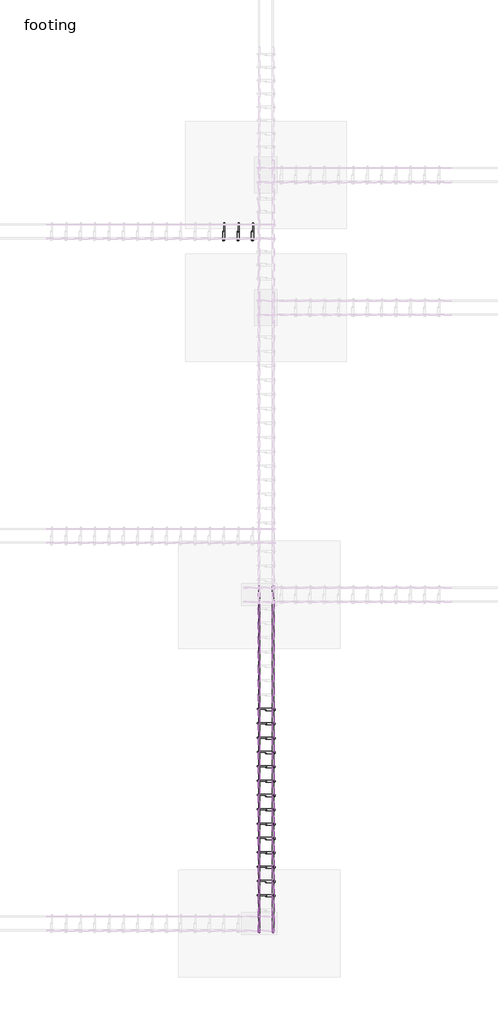
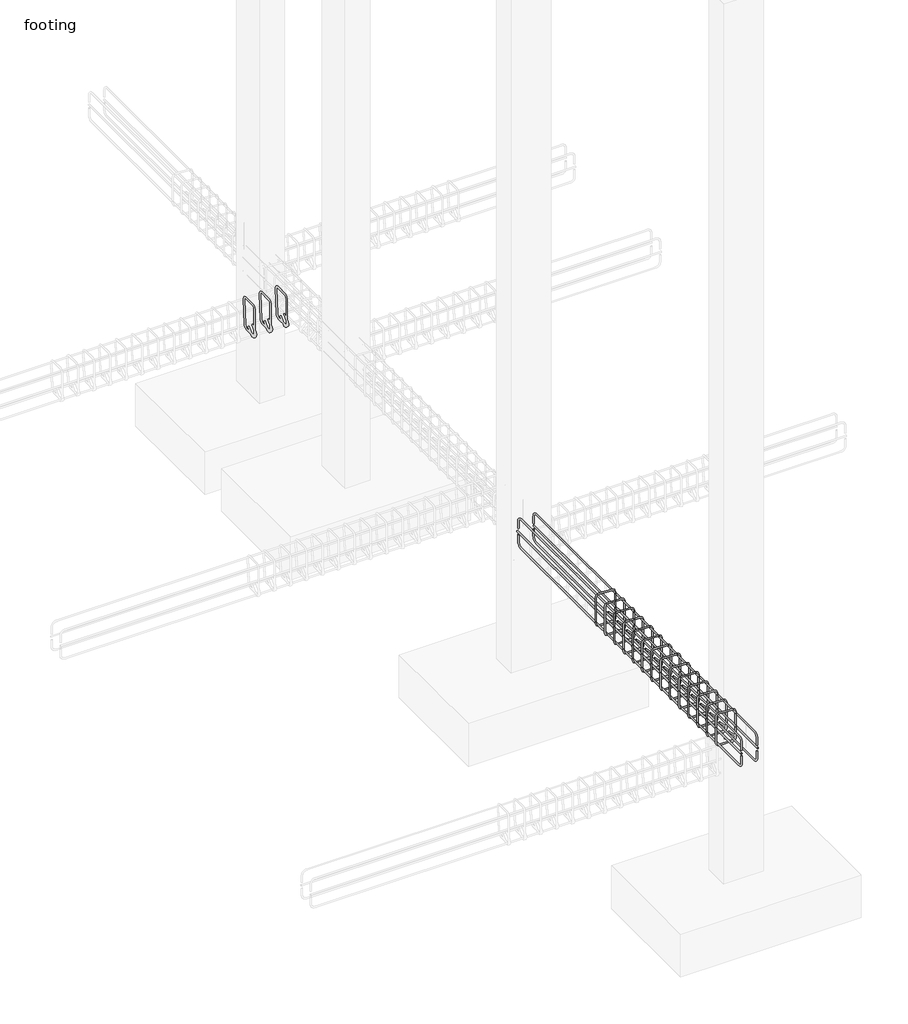
# One storey, part 9 of 21: 23 reinforcing bars.
"""IFC4 building model written with IfcOpenShell, lengths in millimetres."""

from ifc_helpers import new_model, si_unit, point, frame, origin, place, context, project, spatial, polyline, circle_curve, trimmed, segment, composite_curve, element, save
from ifc_brep_helpers import swept_disk

model = new_model("IFC4")

# Units and contexts
model_context = context("Model", 3, world=origin())
ifc_project = project(units=[si_unit("LENGTHUNIT", "METRE", prefix="MILLI")], contexts=[model_context])

# Site, building, storey
site = spatial("IfcSite", under=ifc_project)
building = spatial("IfcBuilding", under=site)
storey = spatial("IfcBuildingStorey", under=building, Name="footing", Elevation=-1524.0)

# Reinforcing bars
placement = place(None, origin())
element("IfcReinforcingBar", 1, at=placement, inside=storey, context=model_context, shape_type="SolidModel", body=[
    swept_disk(composite_curve([segment(polyline([(-8352.8883428, 7572.2887132, -310.8825168), (-8352.8883428, 7517.4237147, -365.7475153)]), True, "CONTINUOUS"), segment(trimmed(circle_curve(frame((-8352.8883428, 7494.9730744, -343.296875), z_axis=(-1.0, 0.0, 0.0), x_axis=(0.0, 22.450640300000487, -22.450640299999975)), 31.75), [point((-8352.8883428, 7517.4237147, -365.7475153))], [point((-8352.8883428, 7463.2230744, -343.296875))], True, "CARTESIAN"), True, "CONTINUOUS"), segment(polyline([(-8352.8883428, 7463.2230744, -343.296875), (-8352.8883428, 7463.2230744, -63.103125)]), True, "CONTINUOUS"), segment(trimmed(circle_curve(frame((-8352.8883428, 7494.9730744, -63.103125), z_axis=(-1.0, 0.0, 0.0), x_axis=(0.0, -31.75, 0.0)), 31.75), [point((-8352.8883428, 7463.2230744, -63.103125))], [point((-8352.8883428, 7494.9730744, -31.353125))], True, "CARTESIAN"), True, "CONTINUOUS"), segment(polyline([(-8352.8883428, 7494.9730744, -31.353125), (-8352.8883428, 7622.7668244, -31.353125)]), True, "CONTINUOUS"), segment(trimmed(circle_curve(frame((-8351.7159328, 7622.7668244, -63.0814712), z_axis=(-0.9993179916193466, 0.0, -0.03692629992126919), x_axis=(-1.1724100000010367, 0.0, 31.728346200000004)), 31.75), [point((-8352.8883428, 7622.7668244, -31.353125))], [point((-8351.7159328, 7654.5168244, -63.0814712))], True, "CARTESIAN"), True, "CONTINUOUS"), segment(polyline([(-8351.7159328, 7654.5168244, -63.0814712), (-8341.3607528, 7654.5168244, -343.3185288)]), True, "CONTINUOUS"), segment(trimmed(circle_curve(frame((-8341.3607528, 7622.7668244, -343.3185288), z_axis=(-0.9993179916193466, 0.0, -0.03692629992126919), x_axis=(0.0, 31.75, 0.0)), 31.75), [point((-8341.3607528, 7654.5168244, -343.3185288))], [point((-8340.1883428, 7622.7668244, -375.046875))], True, "CARTESIAN"), True, "CONTINUOUS"), segment(polyline([(-8340.1883428, 7622.7668244, -375.046875), (-8340.1883428, 7494.9730744, -375.046875)]), True, "CONTINUOUS"), segment(trimmed(circle_curve(frame((-8340.1883428, 7494.9730744, -343.296875), z_axis=(-1.0, 0.0, 0.0), x_axis=(0.0, 0.0, -31.75)), 31.75), [point((-8340.1883428, 7494.9730744, -375.046875))], [point((-8340.1883428, 7472.5224341, -320.8462347))], True, "CARTESIAN"), True, "CONTINUOUS"), segment(polyline([(-8340.1883428, 7472.5224341, -320.8462347), (-8340.1883428, 7527.3874326, -265.9812362)]), True, "CONTINUOUS")], self_intersect=False), 6.35),
])
element("IfcReinforcingBar", 2, at=placement, inside=storey, context=model_context, shape_type="SolidModel", body=[
    swept_disk(composite_curve([segment(polyline([(-8190.1883428, 7572.2887132, -310.8825168), (-8190.1883428, 7517.4237147, -365.7475153)]), True, "CONTINUOUS"), segment(trimmed(circle_curve(frame((-8190.1883428, 7494.9730744, -343.296875), z_axis=(-1.0, 0.0, 0.0), x_axis=(0.0, 22.450640300000487, -22.450640299999975)), 31.75), [point((-8190.1883428, 7517.4237147, -365.7475153))], [point((-8190.1883428, 7463.2230744, -343.296875))], True, "CARTESIAN"), True, "CONTINUOUS"), segment(polyline([(-8190.1883428, 7463.2230744, -343.296875), (-8190.1883428, 7463.2230744, -63.103125)]), True, "CONTINUOUS"), segment(trimmed(circle_curve(frame((-8190.1883428, 7494.9730744, -63.103125), z_axis=(-1.0, 0.0, 0.0), x_axis=(0.0, -31.75, 0.0)), 31.75), [point((-8190.1883428, 7463.2230744, -63.103125))], [point((-8190.1883428, 7494.9730744, -31.353125))], True, "CARTESIAN"), True, "CONTINUOUS"), segment(polyline([(-8190.1883428, 7494.9730744, -31.353125), (-8190.1883428, 7622.7668244, -31.353125)]), True, "CONTINUOUS"), segment(trimmed(circle_curve(frame((-8189.0159328, 7622.7668244, -63.0814712), z_axis=(-0.9993179916193466, 0.0, -0.03692629992126919), x_axis=(-1.1724100000001272, 0.0, 31.728346200000004)), 31.75), [point((-8190.1883428, 7622.7668244, -31.353125))], [point((-8189.0159328, 7654.5168244, -63.0814712))], True, "CARTESIAN"), True, "CONTINUOUS"), segment(polyline([(-8189.0159328, 7654.5168244, -63.0814712), (-8178.6607528, 7654.5168244, -343.3185288)]), True, "CONTINUOUS"), segment(trimmed(circle_curve(frame((-8178.6607528, 7622.7668244, -343.3185288), z_axis=(-0.9993179916193466, 0.0, -0.03692629992126919), x_axis=(0.0, 31.75, 0.0)), 31.75), [point((-8178.6607528, 7654.5168244, -343.3185288))], [point((-8177.4883428, 7622.7668244, -375.046875))], True, "CARTESIAN"), True, "CONTINUOUS"), segment(polyline([(-8177.4883428, 7622.7668244, -375.046875), (-8177.4883428, 7494.9730744, -375.046875)]), True, "CONTINUOUS"), segment(trimmed(circle_curve(frame((-8177.4883428, 7494.9730744, -343.296875), z_axis=(-1.0, 0.0, 0.0), x_axis=(0.0, 0.0, -31.75)), 31.75), [point((-8177.4883428, 7494.9730744, -375.046875))], [point((-8177.4883428, 7472.5224341, -320.8462347))], True, "CARTESIAN"), True, "CONTINUOUS"), segment(polyline([(-8177.4883428, 7472.5224341, -320.8462347), (-8177.4883428, 7527.3874326, -265.9812362)]), True, "CONTINUOUS")], self_intersect=False), 6.35),
])
element("IfcReinforcingBar", 3, at=placement, inside=storey, context=model_context, shape_type="SolidModel", body=[
    swept_disk(composite_curve([segment(polyline([(-8027.4883428, 7572.2887132, -310.8825168), (-8027.4883428, 7517.4237147, -365.7475153)]), True, "CONTINUOUS"), segment(trimmed(circle_curve(frame((-8027.4883428, 7494.9730744, -343.296875), z_axis=(-1.0, 0.0, 0.0), x_axis=(0.0, 22.450640300000487, -22.450640299999975)), 31.75), [point((-8027.4883428, 7517.4237147, -365.7475153))], [point((-8027.4883428, 7463.2230744, -343.296875))], True, "CARTESIAN"), True, "CONTINUOUS"), segment(polyline([(-8027.4883428, 7463.2230744, -343.296875), (-8027.4883428, 7463.2230744, -63.103125)]), True, "CONTINUOUS"), segment(trimmed(circle_curve(frame((-8027.4883428, 7494.9730744, -63.103125), z_axis=(-1.0, 0.0, 0.0), x_axis=(0.0, -31.75, 0.0)), 31.75), [point((-8027.4883428, 7463.2230744, -63.103125))], [point((-8027.4883428, 7494.9730744, -31.353125))], True, "CARTESIAN"), True, "CONTINUOUS"), segment(polyline([(-8027.4883428, 7494.9730744, -31.353125), (-8027.4883428, 7622.7668244, -31.353125)]), True, "CONTINUOUS"), segment(trimmed(circle_curve(frame((-8026.3159328, 7622.7668244, -63.0814712), z_axis=(-0.9993179916193466, 0.0, -0.03692629992126919), x_axis=(-1.1724100000001272, 0.0, 31.728346200000004)), 31.75), [point((-8027.4883428, 7622.7668244, -31.353125))], [point((-8026.3159328, 7654.5168244, -63.0814712))], True, "CARTESIAN"), True, "CONTINUOUS"), segment(polyline([(-8026.3159328, 7654.5168244, -63.0814712), (-8015.9607528, 7654.5168244, -343.3185288)]), True, "CONTINUOUS"), segment(trimmed(circle_curve(frame((-8015.9607528, 7622.7668244, -343.3185288), z_axis=(-0.9993179916193466, 0.0, -0.03692629992126919), x_axis=(0.0, 31.75, 0.0)), 31.75), [point((-8015.9607528, 7654.5168244, -343.3185288))], [point((-8014.7883428, 7622.7668244, -375.046875))], True, "CARTESIAN"), True, "CONTINUOUS"), segment(polyline([(-8014.7883428, 7622.7668244, -375.046875), (-8014.7883428, 7494.9730744, -375.046875)]), True, "CONTINUOUS"), segment(trimmed(circle_curve(frame((-8014.7883428, 7494.9730744, -343.296875), z_axis=(-1.0, 0.0, 0.0), x_axis=(0.0, 0.0, -31.75)), 31.75), [point((-8014.7883428, 7494.9730744, -375.046875))], [point((-8014.7883428, 7472.5224341, -320.8462347))], True, "CARTESIAN"), True, "CONTINUOUS"), segment(polyline([(-8014.7883428, 7472.5224341, -320.8462347), (-8014.7883428, 7527.3874326, -265.9812362)]), True, "CONTINUOUS")], self_intersect=False), 6.35),
])
element("IfcReinforcingBar", 4, at=placement, inside=storey, context=model_context, shape_type="SolidModel", body=[
    swept_disk(composite_curve([segment(polyline([(-7834.7165254, 26.8956073, -265.9812362), (-7779.851527, 26.8956073, -320.8462347)]), True, "CONTINUOUS"), segment(trimmed(circle_curve(frame((-7802.3021673, 26.8956073, -343.296875), z_axis=(0.0, 1.0, 0.0), x_axis=(22.450640300000487, 0.0, 22.450640299999975)), 31.75), [point((-7779.851527, 26.8956073, -320.8462347))], [point((-7802.3021673, 26.8956073, -375.046875))], True, "CARTESIAN"), True, "CONTINUOUS"), segment(polyline([(-7802.3021673, 26.8956073, -375.046875), (-7930.0959173, 26.8956073, -375.046875)]), True, "CONTINUOUS"), segment(trimmed(circle_curve(frame((-7930.0959173, 26.8956073, -343.296875), z_axis=(0.0, 1.0, 0.0), x_axis=(0.0, 0.0, -31.75)), 31.75), [point((-7930.0959173, 26.8956073, -375.046875))], [point((-7961.8459173, 26.8956073, -343.296875))], True, "CARTESIAN"), True, "CONTINUOUS"), segment(polyline([(-7961.8459173, 26.8956073, -343.296875), (-7961.8459173, 26.8956073, -63.103125)]), True, "CONTINUOUS"), segment(trimmed(circle_curve(frame((-7930.165658, 24.7923536, -63.103125), z_axis=(0.0662442117686417, 0.9978034397651431, 0.0), x_axis=(-31.680259300000216, 2.1032537000000033, 0.0)), 31.75), [point((-7961.8459173, 26.8956073, -63.103125))], [point((-7930.165658, 24.7923536, -31.353125))], True, "CARTESIAN"), True, "CONTINUOUS"), segment(polyline([(-7930.165658, 24.7923536, -31.353125), (-7802.2324265, 16.298861, -31.353125)]), True, "CONTINUOUS"), segment(trimmed(circle_curve(frame((-7802.2324265, 16.298861, -63.103125), z_axis=(0.06624421176864169, 0.997803439765143, 0.0), x_axis=(0.0, 0.0, 31.75)), 31.75), [point((-7802.2324265, 16.298861, -31.353125))], [point((-7770.5521673, 14.1956073, -63.103125))], True, "CARTESIAN"), True, "CONTINUOUS"), segment(polyline([(-7770.5521673, 14.1956073, -63.103125), (-7770.5521673, 14.1956073, -343.296875)]), True, "CONTINUOUS"), segment(trimmed(circle_curve(frame((-7802.3021673, 14.1956073, -343.296875), z_axis=(0.0, 1.0, 0.0), x_axis=(31.75, 0.0, 0.0)), 31.75), [point((-7770.5521673, 14.1956073, -343.296875))], [point((-7824.7528076, 14.1956073, -365.7475153))], True, "CARTESIAN"), True, "CONTINUOUS"), segment(polyline([(-7824.7528076, 14.1956073, -365.7475153), (-7879.617806, 14.1956073, -310.8825168)]), True, "CONTINUOUS")], self_intersect=False), 6.35),
])
element("IfcReinforcingBar", 5, at=placement, inside=storey, context=model_context, shape_type="SolidModel", body=[
    swept_disk(composite_curve([segment(polyline([(-7834.7165254, 189.5956073, -265.9812362), (-7779.851527, 189.5956073, -320.8462347)]), True, "CONTINUOUS"), segment(trimmed(circle_curve(frame((-7802.3021673, 189.5956073, -343.296875), z_axis=(0.0, 1.0, 0.0), x_axis=(22.450640300000487, 0.0, 22.450640299999975)), 31.75), [point((-7779.851527, 189.5956073, -320.8462347))], [point((-7802.3021673, 189.5956073, -375.046875))], True, "CARTESIAN"), True, "CONTINUOUS"), segment(polyline([(-7802.3021673, 189.5956073, -375.046875), (-7930.0959173, 189.5956073, -375.046875)]), True, "CONTINUOUS"), segment(trimmed(circle_curve(frame((-7930.0959173, 189.5956073, -343.296875), z_axis=(0.0, 1.0, 0.0), x_axis=(0.0, 0.0, -31.75)), 31.75), [point((-7930.0959173, 189.5956073, -375.046875))], [point((-7961.8459173, 189.5956073, -343.296875))], True, "CARTESIAN"), True, "CONTINUOUS"), segment(polyline([(-7961.8459173, 189.5956073, -343.296875), (-7961.8459173, 189.5956073, -63.103125)]), True, "CONTINUOUS"), segment(trimmed(circle_curve(frame((-7930.165658, 187.4923536, -63.103125), z_axis=(0.0662442117686417, 0.9978034397651431, 0.0), x_axis=(-31.680259300000216, 2.1032537000000104, 0.0)), 31.75), [point((-7961.8459173, 189.5956073, -63.103125))], [point((-7930.165658, 187.4923536, -31.353125))], True, "CARTESIAN"), True, "CONTINUOUS"), segment(polyline([(-7930.165658, 187.4923536, -31.353125), (-7802.2324265, 178.998861, -31.353125)]), True, "CONTINUOUS"), segment(trimmed(circle_curve(frame((-7802.2324265, 178.998861, -63.103125), z_axis=(0.06624421176864169, 0.997803439765143, 0.0), x_axis=(0.0, 0.0, 31.75)), 31.75), [point((-7802.2324265, 178.998861, -31.353125))], [point((-7770.5521673, 176.8956073, -63.103125))], True, "CARTESIAN"), True, "CONTINUOUS"), segment(polyline([(-7770.5521673, 176.8956073, -63.103125), (-7770.5521673, 176.8956073, -343.296875)]), True, "CONTINUOUS"), segment(trimmed(circle_curve(frame((-7802.3021673, 176.8956073, -343.296875), z_axis=(0.0, 1.0, 0.0), x_axis=(31.75, 0.0, 0.0)), 31.75), [point((-7770.5521673, 176.8956073, -343.296875))], [point((-7824.7528076, 176.8956073, -365.7475153))], True, "CARTESIAN"), True, "CONTINUOUS"), segment(polyline([(-7824.7528076, 176.8956073, -365.7475153), (-7879.617806, 176.8956073, -310.8825168)]), True, "CONTINUOUS")], self_intersect=False), 6.35),
])
element("IfcReinforcingBar", 6, at=placement, inside=storey, context=model_context, shape_type="SolidModel", body=[
    swept_disk(composite_curve([segment(polyline([(-7834.7165254, 352.2956073, -265.9812362), (-7779.851527, 352.2956073, -320.8462347)]), True, "CONTINUOUS"), segment(trimmed(circle_curve(frame((-7802.3021673, 352.2956073, -343.296875), z_axis=(0.0, 1.0, 0.0), x_axis=(22.450640300000487, 0.0, 22.450640299999975)), 31.75), [point((-7779.851527, 352.2956073, -320.8462347))], [point((-7802.3021673, 352.2956073, -375.046875))], True, "CARTESIAN"), True, "CONTINUOUS"), segment(polyline([(-7802.3021673, 352.2956073, -375.046875), (-7930.0959173, 352.2956073, -375.046875)]), True, "CONTINUOUS"), segment(trimmed(circle_curve(frame((-7930.0959173, 352.2956073, -343.296875), z_axis=(0.0, 1.0, 0.0), x_axis=(0.0, 0.0, -31.75)), 31.75), [point((-7930.0959173, 352.2956073, -375.046875))], [point((-7961.8459173, 352.2956073, -343.296875))], True, "CARTESIAN"), True, "CONTINUOUS"), segment(polyline([(-7961.8459173, 352.2956073, -343.296875), (-7961.8459173, 352.2956073, -63.103125)]), True, "CONTINUOUS"), segment(trimmed(circle_curve(frame((-7930.165658, 350.1923536, -63.103125), z_axis=(0.0662442117686417, 0.9978034397651431, 0.0), x_axis=(-31.680259300000216, 2.103253699999982, 0.0)), 31.75), [point((-7961.8459173, 352.2956073, -63.103125))], [point((-7930.165658, 350.1923536, -31.353125))], True, "CARTESIAN"), True, "CONTINUOUS"), segment(polyline([(-7930.165658, 350.1923536, -31.353125), (-7802.2324265, 341.698861, -31.353125)]), True, "CONTINUOUS"), segment(trimmed(circle_curve(frame((-7802.2324265, 341.698861, -63.103125), z_axis=(0.06624421176864169, 0.997803439765143, 0.0), x_axis=(0.0, 0.0, 31.75)), 31.75), [point((-7802.2324265, 341.698861, -31.353125))], [point((-7770.5521673, 339.5956073, -63.103125))], True, "CARTESIAN"), True, "CONTINUOUS"), segment(polyline([(-7770.5521673, 339.5956073, -63.103125), (-7770.5521673, 339.5956073, -343.296875)]), True, "CONTINUOUS"), segment(trimmed(circle_curve(frame((-7802.3021673, 339.5956073, -343.296875), z_axis=(0.0, 1.0, 0.0), x_axis=(31.75, 0.0, 0.0)), 31.75), [point((-7770.5521673, 339.5956073, -343.296875))], [point((-7824.7528076, 339.5956073, -365.7475153))], True, "CARTESIAN"), True, "CONTINUOUS"), segment(polyline([(-7824.7528076, 339.5956073, -365.7475153), (-7879.617806, 339.5956073, -310.8825168)]), True, "CONTINUOUS")], self_intersect=False), 6.35),
])
element("IfcReinforcingBar", 7, at=placement, inside=storey, context=model_context, shape_type="SolidModel", body=[
    swept_disk(composite_curve([segment(polyline([(-7834.7165254, 514.9956073, -265.9812362), (-7779.851527, 514.9956073, -320.8462347)]), True, "CONTINUOUS"), segment(trimmed(circle_curve(frame((-7802.3021673, 514.9956073, -343.296875), z_axis=(0.0, 1.0, 0.0), x_axis=(22.450640300000487, 0.0, 22.450640299999975)), 31.75), [point((-7779.851527, 514.9956073, -320.8462347))], [point((-7802.3021673, 514.9956073, -375.046875))], True, "CARTESIAN"), True, "CONTINUOUS"), segment(polyline([(-7802.3021673, 514.9956073, -375.046875), (-7930.0959173, 514.9956073, -375.046875)]), True, "CONTINUOUS"), segment(trimmed(circle_curve(frame((-7930.0959173, 514.9956073, -343.296875), z_axis=(0.0, 1.0, 0.0), x_axis=(0.0, 0.0, -31.75)), 31.75), [point((-7930.0959173, 514.9956073, -375.046875))], [point((-7961.8459173, 514.9956073, -343.296875))], True, "CARTESIAN"), True, "CONTINUOUS"), segment(polyline([(-7961.8459173, 514.9956073, -343.296875), (-7961.8459173, 514.9956073, -63.103125)]), True, "CONTINUOUS"), segment(trimmed(circle_curve(frame((-7930.165658, 512.8923536, -63.103125), z_axis=(0.0662442117686417, 0.9978034397651431, 0.0), x_axis=(-31.680259300000216, 2.103253699999982, 0.0)), 31.75), [point((-7961.8459173, 514.9956073, -63.103125))], [point((-7930.165658, 512.8923536, -31.353125))], True, "CARTESIAN"), True, "CONTINUOUS"), segment(polyline([(-7930.165658, 512.8923536, -31.353125), (-7802.2324265, 504.398861, -31.353125)]), True, "CONTINUOUS"), segment(trimmed(circle_curve(frame((-7802.2324265, 504.398861, -63.103125), z_axis=(0.06624421176864169, 0.997803439765143, 0.0), x_axis=(0.0, 0.0, 31.75)), 31.75), [point((-7802.2324265, 504.398861, -31.353125))], [point((-7770.5521673, 502.2956073, -63.103125))], True, "CARTESIAN"), True, "CONTINUOUS"), segment(polyline([(-7770.5521673, 502.2956073, -63.103125), (-7770.5521673, 502.2956073, -343.296875)]), True, "CONTINUOUS"), segment(trimmed(circle_curve(frame((-7802.3021673, 502.2956073, -343.296875), z_axis=(0.0, 1.0, 0.0), x_axis=(31.75, 0.0, 0.0)), 31.75), [point((-7770.5521673, 502.2956073, -343.296875))], [point((-7824.7528076, 502.2956073, -365.7475153))], True, "CARTESIAN"), True, "CONTINUOUS"), segment(polyline([(-7824.7528076, 502.2956073, -365.7475153), (-7879.617806, 502.2956073, -310.8825168)]), True, "CONTINUOUS")], self_intersect=False), 6.35),
])
element("IfcReinforcingBar", 8, at=placement, inside=storey, context=model_context, shape_type="SolidModel", body=[
    swept_disk(composite_curve([segment(polyline([(-7834.7165254, 677.6956073, -265.9812362), (-7779.851527, 677.6956073, -320.8462347)]), True, "CONTINUOUS"), segment(trimmed(circle_curve(frame((-7802.3021673, 677.6956073, -343.296875), z_axis=(0.0, 1.0, 0.0), x_axis=(22.450640300000487, 0.0, 22.450640299999975)), 31.75), [point((-7779.851527, 677.6956073, -320.8462347))], [point((-7802.3021673, 677.6956073, -375.046875))], True, "CARTESIAN"), True, "CONTINUOUS"), segment(polyline([(-7802.3021673, 677.6956073, -375.046875), (-7930.0959173, 677.6956073, -375.046875)]), True, "CONTINUOUS"), segment(trimmed(circle_curve(frame((-7930.0959173, 677.6956073, -343.296875), z_axis=(0.0, 1.0, 0.0), x_axis=(0.0, 0.0, -31.75)), 31.75), [point((-7930.0959173, 677.6956073, -375.046875))], [point((-7961.8459173, 677.6956073, -343.296875))], True, "CARTESIAN"), True, "CONTINUOUS"), segment(polyline([(-7961.8459173, 677.6956073, -343.296875), (-7961.8459173, 677.6956073, -63.103125)]), True, "CONTINUOUS"), segment(trimmed(circle_curve(frame((-7930.165658, 675.5923536, -63.103125), z_axis=(0.0662442117686417, 0.9978034397651431, 0.0), x_axis=(-31.680259300000216, 2.103253699999982, 0.0)), 31.75), [point((-7961.8459173, 677.6956073, -63.103125))], [point((-7930.165658, 675.5923536, -31.353125))], True, "CARTESIAN"), True, "CONTINUOUS"), segment(polyline([(-7930.165658, 675.5923536, -31.353125), (-7802.2324265, 667.098861, -31.353125)]), True, "CONTINUOUS"), segment(trimmed(circle_curve(frame((-7802.2324265, 667.098861, -63.103125), z_axis=(0.06624421176864169, 0.997803439765143, 0.0), x_axis=(0.0, 0.0, 31.75)), 31.75), [point((-7802.2324265, 667.098861, -31.353125))], [point((-7770.5521673, 664.9956073, -63.103125))], True, "CARTESIAN"), True, "CONTINUOUS"), segment(polyline([(-7770.5521673, 664.9956073, -63.103125), (-7770.5521673, 664.9956073, -343.296875)]), True, "CONTINUOUS"), segment(trimmed(circle_curve(frame((-7802.3021673, 664.9956073, -343.296875), z_axis=(0.0, 1.0, 0.0), x_axis=(31.75, 0.0, 0.0)), 31.75), [point((-7770.5521673, 664.9956073, -343.296875))], [point((-7824.7528076, 664.9956073, -365.7475153))], True, "CARTESIAN"), True, "CONTINUOUS"), segment(polyline([(-7824.7528076, 664.9956073, -365.7475153), (-7879.617806, 664.9956073, -310.8825168)]), True, "CONTINUOUS")], self_intersect=False), 6.35),
])
element("IfcReinforcingBar", 9, at=placement, inside=storey, context=model_context, shape_type="SolidModel", body=[
    swept_disk(composite_curve([segment(polyline([(-7834.7165254, 840.3956073, -265.9812362), (-7779.851527, 840.3956073, -320.8462347)]), True, "CONTINUOUS"), segment(trimmed(circle_curve(frame((-7802.3021673, 840.3956073, -343.296875), z_axis=(0.0, 1.0, 0.0), x_axis=(22.450640300000487, 0.0, 22.450640299999975)), 31.75), [point((-7779.851527, 840.3956073, -320.8462347))], [point((-7802.3021673, 840.3956073, -375.046875))], True, "CARTESIAN"), True, "CONTINUOUS"), segment(polyline([(-7802.3021673, 840.3956073, -375.046875), (-7930.0959173, 840.3956073, -375.046875)]), True, "CONTINUOUS"), segment(trimmed(circle_curve(frame((-7930.0959173, 840.3956073, -343.296875), z_axis=(0.0, 1.0, 0.0), x_axis=(0.0, 0.0, -31.75)), 31.75), [point((-7930.0959173, 840.3956073, -375.046875))], [point((-7961.8459173, 840.3956073, -343.296875))], True, "CARTESIAN"), True, "CONTINUOUS"), segment(polyline([(-7961.8459173, 840.3956073, -343.296875), (-7961.8459173, 840.3956073, -63.103125)]), True, "CONTINUOUS"), segment(trimmed(circle_curve(frame((-7930.165658, 838.2923536, -63.103125), z_axis=(0.0662442117686417, 0.9978034397651431, 0.0), x_axis=(-31.680259300000216, 2.1032537000000957, 0.0)), 31.75), [point((-7961.8459173, 840.3956073, -63.103125))], [point((-7930.165658, 838.2923536, -31.353125))], True, "CARTESIAN"), True, "CONTINUOUS"), segment(polyline([(-7930.165658, 838.2923536, -31.353125), (-7802.2324265, 829.798861, -31.353125)]), True, "CONTINUOUS"), segment(trimmed(circle_curve(frame((-7802.2324265, 829.798861, -63.103125), z_axis=(0.06624421176864169, 0.997803439765143, 0.0), x_axis=(0.0, 0.0, 31.75)), 31.75), [point((-7802.2324265, 829.798861, -31.353125))], [point((-7770.5521673, 827.6956073, -63.103125))], True, "CARTESIAN"), True, "CONTINUOUS"), segment(polyline([(-7770.5521673, 827.6956073, -63.103125), (-7770.5521673, 827.6956073, -343.296875)]), True, "CONTINUOUS"), segment(trimmed(circle_curve(frame((-7802.3021673, 827.6956073, -343.296875), z_axis=(0.0, 1.0, 0.0), x_axis=(31.75, 0.0, 0.0)), 31.75), [point((-7770.5521673, 827.6956073, -343.296875))], [point((-7824.7528076, 827.6956073, -365.7475153))], True, "CARTESIAN"), True, "CONTINUOUS"), segment(polyline([(-7824.7528076, 827.6956073, -365.7475153), (-7879.617806, 827.6956073, -310.8825168)]), True, "CONTINUOUS")], self_intersect=False), 6.35),
])
element("IfcReinforcingBar", 10, at=placement, inside=storey, context=model_context, shape_type="SolidModel", body=[
    swept_disk(composite_curve([segment(polyline([(-7834.7165254, 1003.0956073, -265.9812362), (-7779.851527, 1003.0956073, -320.8462347)]), True, "CONTINUOUS"), segment(trimmed(circle_curve(frame((-7802.3021673, 1003.0956073, -343.296875), z_axis=(0.0, 1.0, 0.0), x_axis=(22.450640300000487, 0.0, 22.450640299999975)), 31.75), [point((-7779.851527, 1003.0956073, -320.8462347))], [point((-7802.3021673, 1003.0956073, -375.046875))], True, "CARTESIAN"), True, "CONTINUOUS"), segment(polyline([(-7802.3021673, 1003.0956073, -375.046875), (-7930.0959173, 1003.0956073, -375.046875)]), True, "CONTINUOUS"), segment(trimmed(circle_curve(frame((-7930.0959173, 1003.0956073, -343.296875), z_axis=(0.0, 1.0, 0.0), x_axis=(0.0, 0.0, -31.75)), 31.75), [point((-7930.0959173, 1003.0956073, -375.046875))], [point((-7961.8459173, 1003.0956073, -343.296875))], True, "CARTESIAN"), True, "CONTINUOUS"), segment(polyline([(-7961.8459173, 1003.0956073, -343.296875), (-7961.8459173, 1003.0956073, -63.103125)]), True, "CONTINUOUS"), segment(trimmed(circle_curve(frame((-7930.165658, 1000.9923536, -63.103125), z_axis=(0.0662442117686417, 0.9978034397651431, 0.0), x_axis=(-31.680259300000216, 2.103253699999982, 0.0)), 31.75), [point((-7961.8459173, 1003.0956073, -63.103125))], [point((-7930.165658, 1000.9923536, -31.353125))], True, "CARTESIAN"), True, "CONTINUOUS"), segment(polyline([(-7930.165658, 1000.9923536, -31.353125), (-7802.2324265, 992.498861, -31.353125)]), True, "CONTINUOUS"), segment(trimmed(circle_curve(frame((-7802.2324265, 992.498861, -63.103125), z_axis=(0.06624421176864169, 0.997803439765143, 0.0), x_axis=(0.0, 0.0, 31.75)), 31.75), [point((-7802.2324265, 992.498861, -31.353125))], [point((-7770.5521673, 990.3956073, -63.103125))], True, "CARTESIAN"), True, "CONTINUOUS"), segment(polyline([(-7770.5521673, 990.3956073, -63.103125), (-7770.5521673, 990.3956073, -343.296875)]), True, "CONTINUOUS"), segment(trimmed(circle_curve(frame((-7802.3021673, 990.3956073, -343.296875), z_axis=(0.0, 1.0, 0.0), x_axis=(31.75, 0.0, 0.0)), 31.75), [point((-7770.5521673, 990.3956073, -343.296875))], [point((-7824.7528076, 990.3956073, -365.7475153))], True, "CARTESIAN"), True, "CONTINUOUS"), segment(polyline([(-7824.7528076, 990.3956073, -365.7475153), (-7879.617806, 990.3956073, -310.8825168)]), True, "CONTINUOUS")], self_intersect=False), 6.35),
])
element("IfcReinforcingBar", 11, at=placement, inside=storey, context=model_context, shape_type="SolidModel", body=[
    swept_disk(composite_curve([segment(polyline([(-7834.7165254, 1165.7956073, -265.9812362), (-7779.851527, 1165.7956073, -320.8462347)]), True, "CONTINUOUS"), segment(trimmed(circle_curve(frame((-7802.3021673, 1165.7956073, -343.296875), z_axis=(0.0, 1.0, 0.0), x_axis=(22.450640300000487, 0.0, 22.450640299999975)), 31.75), [point((-7779.851527, 1165.7956073, -320.8462347))], [point((-7802.3021673, 1165.7956073, -375.046875))], True, "CARTESIAN"), True, "CONTINUOUS"), segment(polyline([(-7802.3021673, 1165.7956073, -375.046875), (-7930.0959173, 1165.7956073, -375.046875)]), True, "CONTINUOUS"), segment(trimmed(circle_curve(frame((-7930.0959173, 1165.7956073, -343.296875), z_axis=(0.0, 1.0, 0.0), x_axis=(0.0, 0.0, -31.75)), 31.75), [point((-7930.0959173, 1165.7956073, -375.046875))], [point((-7961.8459173, 1165.7956073, -343.296875))], True, "CARTESIAN"), True, "CONTINUOUS"), segment(polyline([(-7961.8459173, 1165.7956073, -343.296875), (-7961.8459173, 1165.7956073, -63.103125)]), True, "CONTINUOUS"), segment(trimmed(circle_curve(frame((-7930.165658, 1163.6923536, -63.103125), z_axis=(0.0662442117686417, 0.9978034397651431, 0.0), x_axis=(-31.680259300000216, 2.1032537000000957, 0.0)), 31.75), [point((-7961.8459173, 1165.7956073, -63.103125))], [point((-7930.165658, 1163.6923536, -31.353125))], True, "CARTESIAN"), True, "CONTINUOUS"), segment(polyline([(-7930.165658, 1163.6923536, -31.353125), (-7802.2324265, 1155.198861, -31.353125)]), True, "CONTINUOUS"), segment(trimmed(circle_curve(frame((-7802.2324265, 1155.198861, -63.103125), z_axis=(0.06624421176864169, 0.997803439765143, 0.0), x_axis=(0.0, 0.0, 31.75)), 31.75), [point((-7802.2324265, 1155.198861, -31.353125))], [point((-7770.5521673, 1153.0956073, -63.103125))], True, "CARTESIAN"), True, "CONTINUOUS"), segment(polyline([(-7770.5521673, 1153.0956073, -63.103125), (-7770.5521673, 1153.0956073, -343.296875)]), True, "CONTINUOUS"), segment(trimmed(circle_curve(frame((-7802.3021673, 1153.0956073, -343.296875), z_axis=(0.0, 1.0, 0.0), x_axis=(31.75, 0.0, 0.0)), 31.75), [point((-7770.5521673, 1153.0956073, -343.296875))], [point((-7824.7528076, 1153.0956073, -365.7475153))], True, "CARTESIAN"), True, "CONTINUOUS"), segment(polyline([(-7824.7528076, 1153.0956073, -365.7475153), (-7879.617806, 1153.0956073, -310.8825168)]), True, "CONTINUOUS")], self_intersect=False), 6.35),
])
element("IfcReinforcingBar", 12, at=placement, inside=storey, context=model_context, shape_type="SolidModel", body=[
    swept_disk(composite_curve([segment(polyline([(-7834.7165254, 1328.4956073, -265.9812362), (-7779.851527, 1328.4956073, -320.8462347)]), True, "CONTINUOUS"), segment(trimmed(circle_curve(frame((-7802.3021673, 1328.4956073, -343.296875), z_axis=(0.0, 1.0, 0.0), x_axis=(22.450640300000487, 0.0, 22.450640299999975)), 31.75), [point((-7779.851527, 1328.4956073, -320.8462347))], [point((-7802.3021673, 1328.4956073, -375.046875))], True, "CARTESIAN"), True, "CONTINUOUS"), segment(polyline([(-7802.3021673, 1328.4956073, -375.046875), (-7930.0959173, 1328.4956073, -375.046875)]), True, "CONTINUOUS"), segment(trimmed(circle_curve(frame((-7930.0959173, 1328.4956073, -343.296875), z_axis=(0.0, 1.0, 0.0), x_axis=(0.0, 0.0, -31.75)), 31.75), [point((-7930.0959173, 1328.4956073, -375.046875))], [point((-7961.8459173, 1328.4956073, -343.296875))], True, "CARTESIAN"), True, "CONTINUOUS"), segment(polyline([(-7961.8459173, 1328.4956073, -343.296875), (-7961.8459173, 1328.4956073, -63.103125)]), True, "CONTINUOUS"), segment(trimmed(circle_curve(frame((-7930.165658, 1326.3923536, -63.103125), z_axis=(0.0662442117686417, 0.9978034397651431, 0.0), x_axis=(-31.680259300000216, 2.1032537000000957, 0.0)), 31.75), [point((-7961.8459173, 1328.4956073, -63.103125))], [point((-7930.165658, 1326.3923536, -31.353125))], True, "CARTESIAN"), True, "CONTINUOUS"), segment(polyline([(-7930.165658, 1326.3923536, -31.353125), (-7802.2324265, 1317.898861, -31.353125)]), True, "CONTINUOUS"), segment(trimmed(circle_curve(frame((-7802.2324265, 1317.898861, -63.103125), z_axis=(0.06624421176864169, 0.997803439765143, 0.0), x_axis=(0.0, 0.0, 31.75)), 31.75), [point((-7802.2324265, 1317.898861, -31.353125))], [point((-7770.5521673, 1315.7956073, -63.103125))], True, "CARTESIAN"), True, "CONTINUOUS"), segment(polyline([(-7770.5521673, 1315.7956073, -63.103125), (-7770.5521673, 1315.7956073, -343.296875)]), True, "CONTINUOUS"), segment(trimmed(circle_curve(frame((-7802.3021673, 1315.7956073, -343.296875), z_axis=(0.0, 1.0, 0.0), x_axis=(31.75, 0.0, 0.0)), 31.75), [point((-7770.5521673, 1315.7956073, -343.296875))], [point((-7824.7528076, 1315.7956073, -365.7475153))], True, "CARTESIAN"), True, "CONTINUOUS"), segment(polyline([(-7824.7528076, 1315.7956073, -365.7475153), (-7879.617806, 1315.7956073, -310.8825168)]), True, "CONTINUOUS")], self_intersect=False), 6.35),
])
element("IfcReinforcingBar", 13, at=placement, inside=storey, context=model_context, shape_type="SolidModel", body=[
    swept_disk(composite_curve([segment(polyline([(-7834.7165254, 1491.1956073, -265.9812362), (-7779.851527, 1491.1956073, -320.8462347)]), True, "CONTINUOUS"), segment(trimmed(circle_curve(frame((-7802.3021673, 1491.1956073, -343.296875), z_axis=(0.0, 1.0, 0.0), x_axis=(22.450640300000487, 0.0, 22.450640299999975)), 31.75), [point((-7779.851527, 1491.1956073, -320.8462347))], [point((-7802.3021673, 1491.1956073, -375.046875))], True, "CARTESIAN"), True, "CONTINUOUS"), segment(polyline([(-7802.3021673, 1491.1956073, -375.046875), (-7930.0959173, 1491.1956073, -375.046875)]), True, "CONTINUOUS"), segment(trimmed(circle_curve(frame((-7930.0959173, 1491.1956073, -343.296875), z_axis=(0.0, 1.0, 0.0), x_axis=(0.0, 0.0, -31.75)), 31.75), [point((-7930.0959173, 1491.1956073, -375.046875))], [point((-7961.8459173, 1491.1956073, -343.296875))], True, "CARTESIAN"), True, "CONTINUOUS"), segment(polyline([(-7961.8459173, 1491.1956073, -343.296875), (-7961.8459173, 1491.1956073, -63.103125)]), True, "CONTINUOUS"), segment(trimmed(circle_curve(frame((-7930.165658, 1489.0923536, -63.103125), z_axis=(0.0662442117686417, 0.9978034397651431, 0.0), x_axis=(-31.680259300000216, 2.1032536999998683, 0.0)), 31.75), [point((-7961.8459173, 1491.1956073, -63.103125))], [point((-7930.165658, 1489.0923536, -31.353125))], True, "CARTESIAN"), True, "CONTINUOUS"), segment(polyline([(-7930.165658, 1489.0923536, -31.353125), (-7802.2324265, 1480.598861, -31.353125)]), True, "CONTINUOUS"), segment(trimmed(circle_curve(frame((-7802.2324265, 1480.598861, -63.103125), z_axis=(0.06624421176864169, 0.997803439765143, 0.0), x_axis=(0.0, 0.0, 31.75)), 31.75), [point((-7802.2324265, 1480.598861, -31.353125))], [point((-7770.5521673, 1478.4956073, -63.103125))], True, "CARTESIAN"), True, "CONTINUOUS"), segment(polyline([(-7770.5521673, 1478.4956073, -63.103125), (-7770.5521673, 1478.4956073, -343.296875)]), True, "CONTINUOUS"), segment(trimmed(circle_curve(frame((-7802.3021673, 1478.4956073, -343.296875), z_axis=(0.0, 1.0, 0.0), x_axis=(31.75, 0.0, 0.0)), 31.75), [point((-7770.5521673, 1478.4956073, -343.296875))], [point((-7824.7528076, 1478.4956073, -365.7475153))], True, "CARTESIAN"), True, "CONTINUOUS"), segment(polyline([(-7824.7528076, 1478.4956073, -365.7475153), (-7879.617806, 1478.4956073, -310.8825168)]), True, "CONTINUOUS")], self_intersect=False), 6.35),
])
element("IfcReinforcingBar", 14, at=placement, inside=storey, context=model_context, shape_type="SolidModel", body=[
    swept_disk(composite_curve([segment(polyline([(-7834.7165254, 1653.8956073, -265.9812362), (-7779.851527, 1653.8956073, -320.8462347)]), True, "CONTINUOUS"), segment(trimmed(circle_curve(frame((-7802.3021673, 1653.8956073, -343.296875), z_axis=(0.0, 1.0, 0.0), x_axis=(22.450640300000487, 0.0, 22.450640299999975)), 31.75), [point((-7779.851527, 1653.8956073, -320.8462347))], [point((-7802.3021673, 1653.8956073, -375.046875))], True, "CARTESIAN"), True, "CONTINUOUS"), segment(polyline([(-7802.3021673, 1653.8956073, -375.046875), (-7930.0959173, 1653.8956073, -375.046875)]), True, "CONTINUOUS"), segment(trimmed(circle_curve(frame((-7930.0959173, 1653.8956073, -343.296875), z_axis=(0.0, 1.0, 0.0), x_axis=(0.0, 0.0, -31.75)), 31.75), [point((-7930.0959173, 1653.8956073, -375.046875))], [point((-7961.8459173, 1653.8956073, -343.296875))], True, "CARTESIAN"), True, "CONTINUOUS"), segment(polyline([(-7961.8459173, 1653.8956073, -343.296875), (-7961.8459173, 1653.8956073, -63.103125)]), True, "CONTINUOUS"), segment(trimmed(circle_curve(frame((-7930.165658, 1651.7923536, -63.103125), z_axis=(0.0662442117686417, 0.9978034397651431, 0.0), x_axis=(-31.680259300000216, 2.1032536999998683, 0.0)), 31.75), [point((-7961.8459173, 1653.8956073, -63.103125))], [point((-7930.165658, 1651.7923536, -31.353125))], True, "CARTESIAN"), True, "CONTINUOUS"), segment(polyline([(-7930.165658, 1651.7923536, -31.353125), (-7802.2324265, 1643.298861, -31.353125)]), True, "CONTINUOUS"), segment(trimmed(circle_curve(frame((-7802.2324265, 1643.298861, -63.103125), z_axis=(0.06624421176864169, 0.997803439765143, 0.0), x_axis=(0.0, 0.0, 31.75)), 31.75), [point((-7802.2324265, 1643.298861, -31.353125))], [point((-7770.5521673, 1641.1956073, -63.103125))], True, "CARTESIAN"), True, "CONTINUOUS"), segment(polyline([(-7770.5521673, 1641.1956073, -63.103125), (-7770.5521673, 1641.1956073, -343.296875)]), True, "CONTINUOUS"), segment(trimmed(circle_curve(frame((-7802.3021673, 1641.1956073, -343.296875), z_axis=(0.0, 1.0, 0.0), x_axis=(31.75, 0.0, 0.0)), 31.75), [point((-7770.5521673, 1641.1956073, -343.296875))], [point((-7824.7528076, 1641.1956073, -365.7475153))], True, "CARTESIAN"), True, "CONTINUOUS"), segment(polyline([(-7824.7528076, 1641.1956073, -365.7475153), (-7879.617806, 1641.1956073, -310.8825168)]), True, "CONTINUOUS")], self_intersect=False), 6.35),
])
element("IfcReinforcingBar", 15, at=placement, inside=storey, context=model_context, shape_type="SolidModel", body=[
    swept_disk(composite_curve([segment(polyline([(-7834.7165254, 1816.5956073, -265.9812362), (-7779.851527, 1816.5956073, -320.8462347)]), True, "CONTINUOUS"), segment(trimmed(circle_curve(frame((-7802.3021673, 1816.5956073, -343.296875), z_axis=(0.0, 1.0, 0.0), x_axis=(22.450640300000487, 0.0, 22.450640299999975)), 31.75), [point((-7779.851527, 1816.5956073, -320.8462347))], [point((-7802.3021673, 1816.5956073, -375.046875))], True, "CARTESIAN"), True, "CONTINUOUS"), segment(polyline([(-7802.3021673, 1816.5956073, -375.046875), (-7930.0959173, 1816.5956073, -375.046875)]), True, "CONTINUOUS"), segment(trimmed(circle_curve(frame((-7930.0959173, 1816.5956073, -343.296875), z_axis=(0.0, 1.0, 0.0), x_axis=(0.0, 0.0, -31.75)), 31.75), [point((-7930.0959173, 1816.5956073, -375.046875))], [point((-7961.8459173, 1816.5956073, -343.296875))], True, "CARTESIAN"), True, "CONTINUOUS"), segment(polyline([(-7961.8459173, 1816.5956073, -343.296875), (-7961.8459173, 1816.5956073, -63.103125)]), True, "CONTINUOUS"), segment(trimmed(circle_curve(frame((-7930.165658, 1814.4923536, -63.103125), z_axis=(0.0662442117686417, 0.9978034397651431, 0.0), x_axis=(-31.680259300000216, 2.1032537000000957, 0.0)), 31.75), [point((-7961.8459173, 1816.5956073, -63.103125))], [point((-7930.165658, 1814.4923536, -31.353125))], True, "CARTESIAN"), True, "CONTINUOUS"), segment(polyline([(-7930.165658, 1814.4923536, -31.353125), (-7802.2324265, 1805.998861, -31.353125)]), True, "CONTINUOUS"), segment(trimmed(circle_curve(frame((-7802.2324265, 1805.998861, -63.103125), z_axis=(0.06624421176864169, 0.997803439765143, 0.0), x_axis=(0.0, 0.0, 31.75)), 31.75), [point((-7802.2324265, 1805.998861, -31.353125))], [point((-7770.5521673, 1803.8956073, -63.103125))], True, "CARTESIAN"), True, "CONTINUOUS"), segment(polyline([(-7770.5521673, 1803.8956073, -63.103125), (-7770.5521673, 1803.8956073, -343.296875)]), True, "CONTINUOUS"), segment(trimmed(circle_curve(frame((-7802.3021673, 1803.8956073, -343.296875), z_axis=(0.0, 1.0, 0.0), x_axis=(31.75, 0.0, 0.0)), 31.75), [point((-7770.5521673, 1803.8956073, -343.296875))], [point((-7824.7528076, 1803.8956073, -365.7475153))], True, "CARTESIAN"), True, "CONTINUOUS"), segment(polyline([(-7824.7528076, 1803.8956073, -365.7475153), (-7879.617806, 1803.8956073, -310.8825168)]), True, "CONTINUOUS")], self_intersect=False), 6.35),
])
element("IfcReinforcingBar", 16, at=placement, inside=storey, context=model_context, shape_type="SolidModel", body=[
    swept_disk(composite_curve([segment(polyline([(-7834.7165254, 1979.2956073, -265.9812362), (-7779.851527, 1979.2956073, -320.8462347)]), True, "CONTINUOUS"), segment(trimmed(circle_curve(frame((-7802.3021673, 1979.2956073, -343.296875), z_axis=(0.0, 1.0, 0.0), x_axis=(22.450640300000487, 0.0, 22.450640299999975)), 31.75), [point((-7779.851527, 1979.2956073, -320.8462347))], [point((-7802.3021673, 1979.2956073, -375.046875))], True, "CARTESIAN"), True, "CONTINUOUS"), segment(polyline([(-7802.3021673, 1979.2956073, -375.046875), (-7930.0959173, 1979.2956073, -375.046875)]), True, "CONTINUOUS"), segment(trimmed(circle_curve(frame((-7930.0959173, 1979.2956073, -343.296875), z_axis=(0.0, 1.0, 0.0), x_axis=(0.0, 0.0, -31.75)), 31.75), [point((-7930.0959173, 1979.2956073, -375.046875))], [point((-7961.8459173, 1979.2956073, -343.296875))], True, "CARTESIAN"), True, "CONTINUOUS"), segment(polyline([(-7961.8459173, 1979.2956073, -343.296875), (-7961.8459173, 1979.2956073, -63.103125)]), True, "CONTINUOUS"), segment(trimmed(circle_curve(frame((-7930.165658, 1977.1923536, -63.103125), z_axis=(0.0662442117686417, 0.9978034397651431, 0.0), x_axis=(-31.680259300000216, 2.1032537000000957, 0.0)), 31.75), [point((-7961.8459173, 1979.2956073, -63.103125))], [point((-7930.165658, 1977.1923536, -31.353125))], True, "CARTESIAN"), True, "CONTINUOUS"), segment(polyline([(-7930.165658, 1977.1923536, -31.353125), (-7802.2324265, 1968.698861, -31.353125)]), True, "CONTINUOUS"), segment(trimmed(circle_curve(frame((-7802.2324265, 1968.698861, -63.103125), z_axis=(0.06624421176864169, 0.997803439765143, 0.0), x_axis=(0.0, 0.0, 31.75)), 31.75), [point((-7802.2324265, 1968.698861, -31.353125))], [point((-7770.5521673, 1966.5956073, -63.103125))], True, "CARTESIAN"), True, "CONTINUOUS"), segment(polyline([(-7770.5521673, 1966.5956073, -63.103125), (-7770.5521673, 1966.5956073, -343.296875)]), True, "CONTINUOUS"), segment(trimmed(circle_curve(frame((-7802.3021673, 1966.5956073, -343.296875), z_axis=(0.0, 1.0, 0.0), x_axis=(31.75, 0.0, 0.0)), 31.75), [point((-7770.5521673, 1966.5956073, -343.296875))], [point((-7824.7528076, 1966.5956073, -365.7475153))], True, "CARTESIAN"), True, "CONTINUOUS"), segment(polyline([(-7824.7528076, 1966.5956073, -365.7475153), (-7879.617806, 1966.5956073, -310.8825168)]), True, "CONTINUOUS")], self_intersect=False), 6.35),
])
element("IfcReinforcingBar", 17, at=placement, inside=storey, context=model_context, shape_type="SolidModel", body=[
    swept_disk(composite_curve([segment(polyline([(-7834.7165254, 2141.9956073, -265.9812362), (-7779.851527, 2141.9956073, -320.8462347)]), True, "CONTINUOUS"), segment(trimmed(circle_curve(frame((-7802.3021673, 2141.9956073, -343.296875), z_axis=(0.0, 1.0, 0.0), x_axis=(22.450640300000487, 0.0, 22.450640299999975)), 31.75), [point((-7779.851527, 2141.9956073, -320.8462347))], [point((-7802.3021673, 2141.9956073, -375.046875))], True, "CARTESIAN"), True, "CONTINUOUS"), segment(polyline([(-7802.3021673, 2141.9956073, -375.046875), (-7930.0959173, 2141.9956073, -375.046875)]), True, "CONTINUOUS"), segment(trimmed(circle_curve(frame((-7930.0959173, 2141.9956073, -343.296875), z_axis=(0.0, 1.0, 0.0), x_axis=(0.0, 0.0, -31.75)), 31.75), [point((-7930.0959173, 2141.9956073, -375.046875))], [point((-7961.8459173, 2141.9956073, -343.296875))], True, "CARTESIAN"), True, "CONTINUOUS"), segment(polyline([(-7961.8459173, 2141.9956073, -343.296875), (-7961.8459173, 2141.9956073, -63.103125)]), True, "CONTINUOUS"), segment(trimmed(circle_curve(frame((-7930.165658, 2139.8923536, -63.103125), z_axis=(0.0662442117686417, 0.9978034397651431, 0.0), x_axis=(-31.680259300000216, 2.103253699999641, 0.0)), 31.75), [point((-7961.8459173, 2141.9956073, -63.103125))], [point((-7930.165658, 2139.8923536, -31.353125))], True, "CARTESIAN"), True, "CONTINUOUS"), segment(polyline([(-7930.165658, 2139.8923536, -31.353125), (-7802.2324265, 2131.398861, -31.353125)]), True, "CONTINUOUS"), segment(trimmed(circle_curve(frame((-7802.2324265, 2131.398861, -63.103125), z_axis=(0.06624421176864169, 0.997803439765143, 0.0), x_axis=(0.0, 0.0, 31.75)), 31.75), [point((-7802.2324265, 2131.398861, -31.353125))], [point((-7770.5521673, 2129.2956073, -63.103125))], True, "CARTESIAN"), True, "CONTINUOUS"), segment(polyline([(-7770.5521673, 2129.2956073, -63.103125), (-7770.5521673, 2129.2956073, -343.296875)]), True, "CONTINUOUS"), segment(trimmed(circle_curve(frame((-7802.3021673, 2129.2956073, -343.296875), z_axis=(0.0, 1.0, 0.0), x_axis=(31.75, 0.0, 0.0)), 31.75), [point((-7770.5521673, 2129.2956073, -343.296875))], [point((-7824.7528076, 2129.2956073, -365.7475153))], True, "CARTESIAN"), True, "CONTINUOUS"), segment(polyline([(-7824.7528076, 2129.2956073, -365.7475153), (-7879.617806, 2129.2956073, -310.8825168)]), True, "CONTINUOUS")], self_intersect=False), 6.35),
])
element("IfcReinforcingBar", 18, at=placement, inside=storey, context=model_context, shape_type="SolidModel", body=[
    swept_disk(composite_curve([segment(polyline([(-7788.8317831, -391.7269256, -170.2827408), (-7788.8317831, -391.7269256, -94.0827408)]), True, "CONTINUOUS"), segment(trimmed(circle_curve(frame((-7788.8317831, -347.2769256, -94.0827408), z_axis=(-1.0, 0.0, 0.0), x_axis=(0.0, -44.44999999999999, 0.0)), 44.45), [point((-7788.8317831, -391.7269256, -94.0827408))], [point((-7788.8317831, -347.2769256, -49.6327408))], True, "CARTESIAN"), True, "CONTINUOUS"), segment(polyline([(-7788.8317831, -347.2769256, -49.6327408), (-7788.8317831, 3488.9168244, -49.6327408)]), True, "CONTINUOUS"), segment(trimmed(circle_curve(frame((-7788.8317831, 3488.9168244, -94.0827408), z_axis=(-1.0, 0.0, 0.0), x_axis=(0.0, 0.0, 44.449999999999996)), 44.45), [point((-7788.8317831, 3488.9168244, -49.6327408))], [point((-7788.8317831, 3533.3668244, -94.0827408))], True, "CARTESIAN"), True, "CONTINUOUS"), segment(polyline([(-7788.8317831, 3533.3668244, -94.0827408), (-7788.8317831, 3533.3668244, -170.2827408)]), True, "CONTINUOUS")], self_intersect=False), 6.35),
])
element("IfcReinforcingBar", 19, at=placement, inside=storey, context=model_context, shape_type="SolidModel", body=[
    swept_disk(composite_curve([segment(polyline([(-7943.5663014, -391.7269256, -170.2827408), (-7943.5663014, -391.7269256, -94.0827408)]), True, "CONTINUOUS"), segment(trimmed(circle_curve(frame((-7943.5663014, -347.2769256, -94.0827408), z_axis=(-1.0, 0.0, 0.0), x_axis=(0.0, -44.44999999999999, 0.0)), 44.45), [point((-7943.5663014, -391.7269256, -94.0827408))], [point((-7943.5663014, -347.2769256, -49.6327408))], True, "CARTESIAN"), True, "CONTINUOUS"), segment(polyline([(-7943.5663014, -347.2769256, -49.6327408), (-7943.5663014, 3488.9168244, -49.6327408)]), True, "CONTINUOUS"), segment(trimmed(circle_curve(frame((-7943.5663014, 3488.9168244, -94.0827408), z_axis=(-1.0, 0.0, 0.0), x_axis=(0.0, 0.0, 44.449999999999996)), 44.45), [point((-7943.5663014, 3488.9168244, -49.6327408))], [point((-7943.5663014, 3533.3668244, -94.0827408))], True, "CARTESIAN"), True, "CONTINUOUS"), segment(polyline([(-7943.5663014, 3533.3668244, -94.0827408), (-7943.5663014, 3533.3668244, -170.2827408)]), True, "CONTINUOUS")], self_intersect=False), 6.35),
])
element("IfcReinforcingBar", 20, at=placement, inside=storey, context=model_context, shape_type="SolidModel", body=[
    swept_disk(composite_curve([segment(polyline([(-7788.8317831, -391.7269256, -236.1172592), (-7788.8317831, -391.7269256, -312.3172592)]), True, "CONTINUOUS"), segment(trimmed(circle_curve(frame((-7788.8317831, -347.2769256, -312.3172592), z_axis=(1.0, 0.0, 0.0), x_axis=(0.0, -44.44999999999999, 0.0)), 44.45), [point((-7788.8317831, -391.7269256, -312.3172592))], [point((-7788.8317831, -347.2769256, -356.7672592))], True, "CARTESIAN"), True, "CONTINUOUS"), segment(polyline([(-7788.8317831, -347.2769256, -356.7672592), (-7788.8317831, 3488.9168244, -356.7672592)]), True, "CONTINUOUS"), segment(trimmed(circle_curve(frame((-7788.8317831, 3488.9168244, -312.3172592), z_axis=(1.0, 0.0, 0.0), x_axis=(0.0, 0.0, -44.44999999999999)), 44.45), [point((-7788.8317831, 3488.9168244, -356.7672592))], [point((-7788.8317831, 3533.3668244, -312.3172592))], True, "CARTESIAN"), True, "CONTINUOUS"), segment(polyline([(-7788.8317831, 3533.3668244, -312.3172592), (-7788.8317831, 3533.3668244, -236.1172592)]), True, "CONTINUOUS")], self_intersect=False), 6.35),
])
element("IfcReinforcingBar", 21, at=placement, inside=storey, context=model_context, shape_type="SolidModel", body=[
    swept_disk(composite_curve([segment(polyline([(-7943.5663014, -391.7269256, -236.1172592), (-7943.5663014, -391.7269256, -312.3172592)]), True, "CONTINUOUS"), segment(trimmed(circle_curve(frame((-7943.5663014, -347.2769256, -312.3172592), z_axis=(1.0, 0.0, 0.0), x_axis=(0.0, -44.44999999999999, 0.0)), 44.45), [point((-7943.5663014, -391.7269256, -312.3172592))], [point((-7943.5663014, -347.2769256, -356.7672592))], True, "CARTESIAN"), True, "CONTINUOUS"), segment(polyline([(-7943.5663014, -347.2769256, -356.7672592), (-7943.5663014, 3488.9168244, -356.7672592)]), True, "CONTINUOUS"), segment(trimmed(circle_curve(frame((-7943.5663014, 3488.9168244, -312.3172592), z_axis=(1.0, 0.0, 0.0), x_axis=(0.0, 0.0, -44.44999999999999)), 44.45), [point((-7943.5663014, 3488.9168244, -356.7672592))], [point((-7943.5663014, 3533.3668244, -312.3172592))], True, "CARTESIAN"), True, "CONTINUOUS"), segment(polyline([(-7943.5663014, 3533.3668244, -312.3172592), (-7943.5663014, 3533.3668244, -236.1172592)]), True, "CONTINUOUS")], self_intersect=False), 6.35),
])
element("IfcReinforcingBar", 22, at=placement, inside=storey, context=model_context, shape_type="SolidModel", body=[
    swept_disk(composite_curve([segment(polyline([(-7783.2521673, -398.0769256, -203.2), (-7783.2521673, 3539.7168244, -203.2)]), True, "CONTINUOUS")], self_intersect=False), 6.35),
])
element("IfcReinforcingBar", 23, at=placement, inside=storey, context=model_context, shape_type="SolidModel", body=[
    swept_disk(composite_curve([segment(polyline([(-7949.1459173, -398.0769256, -203.2), (-7949.1459173, 3539.7168244, -203.2)]), True, "CONTINUOUS")], self_intersect=False), 6.35),
])

save(model, "model.ifc")

# Revit data of these elements
# Elements 1, 2, 3, 4, 5, 6, 7, 8, 9, 10, 11, 12, 13, 14, 15, 16, 17, 18, 19, 20, 21, 22, 23 (IfcReinforcingBar)
#   Phase Created = New Construction
